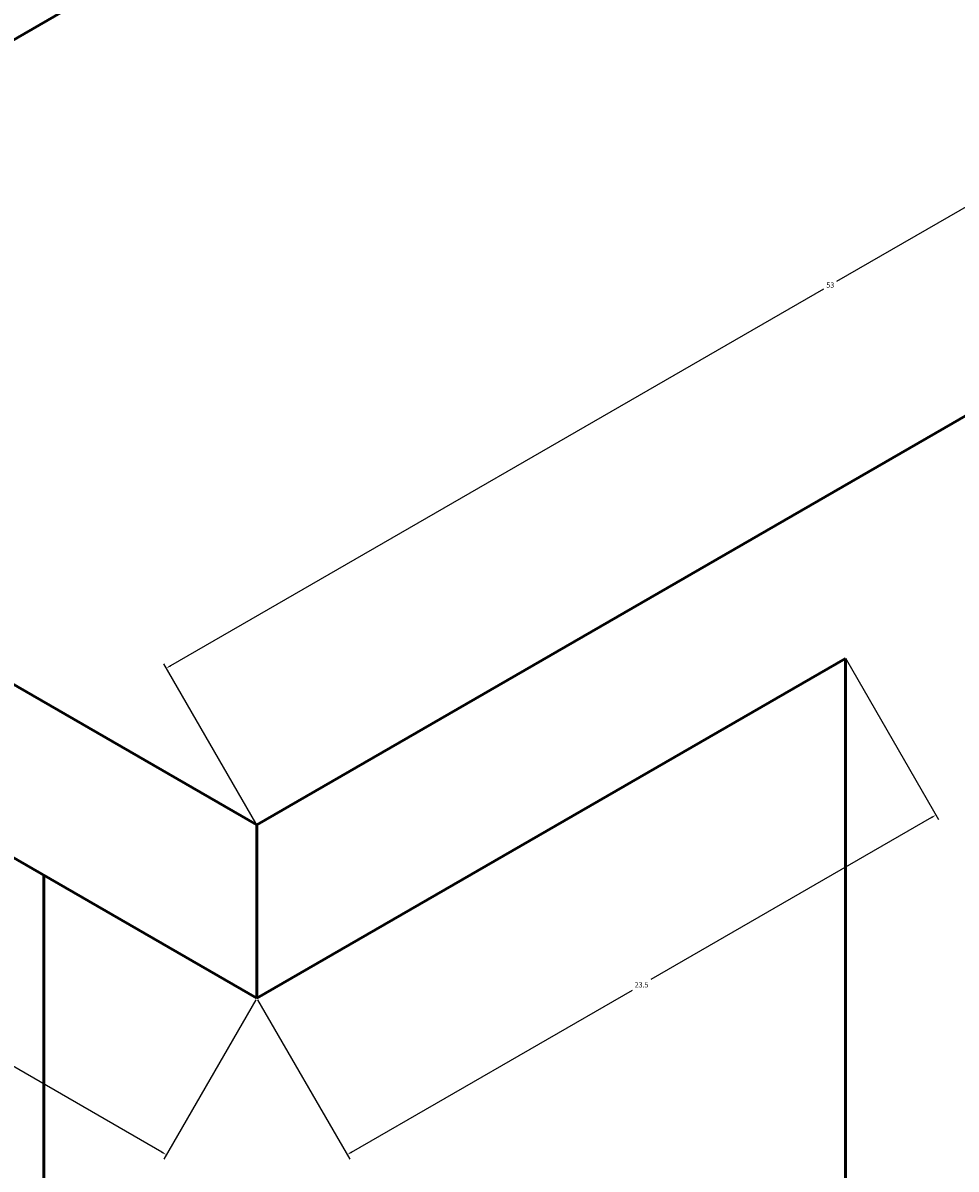
# Model space of a CAD drawing. Units: inches. Extents: x -23 to 69, y -27 to 96.
# Tile 3 of 10: x 8 to 40, y -5 to 35. Entities that reach past the tile are written whole.
import ezdxf

# ---------------------------------------------------------------- set-up
doc = ezdxf.new("R2010")
doc.units = ezdxf.units.IN
doc.header["$MEASUREMENT"] = 0
doc.layers.add('M-DIMS', color=2, linetype='Continuous', lineweight=18)
doc.layers.add('M-OUTL', color=7, linetype='Continuous', lineweight=50)
doc.styles.get("Standard").update_dxf_attribs({"font": 'arial.ttf'})
doc.dimstyles.get("Standard").update_dxf_attribs({"dimtxt": 0.18, "dimasz": 0.18, "dimexe": 0.18, "dimexo": 0.0625, "dimgap": 0.09, "dimtad": 0, "dimtih": 1, "dimtoh": 1, "dimdec": 4, "dimzin": 0, "dimdsep": 46, "dimtxsty": 'Standard', "dimcen": 0.09, "dimadec": 0, "dimazin": 0, "dimtfac": 1, "dimtdec": 4, "dimtofl": 0, "dimtmove": 0, "dimatfit": 3, "dimfxl": 1, "dimtolj": 1, "dimtzin": 0, "dimarcsym": 0})

# ---------------------------------------------------------------- blocks, each defined once
blk = doc.blocks.new('*D1')
at = {"layer": 'Defpoints', "color": 0, "transparency": 16777216}
for p in [(59.046, 39.281), (62.171, 33.869), (16.271, 7.369)]:
    blk.add_point(p, dxfattribs=at)
at = {"layer": 'M-DIMS', "color": 0, "lineweight": -2, "transparency": 16777216}
for p, q in [((62.139, 33.923), (58.956, 39.437)), ((58.89, 39.191), (36.315, 26.158)), ((13.302, 12.871), (35.877, 25.905)), ((16.24, 7.423), (13.056, 12.937))]:
    blk.add_line(p, q, dxfattribs=at)
at = {"layer": 'M-DIMS', "color": 0, "transparency": 16777216}
for points in [[(58.875, 39.217), (58.905, 39.165), (59.046, 39.281)], [(13.287, 12.897), (13.317, 12.845), (13.146, 12.781)]]:
    blk.add_solid(points, dxfattribs=at)
at = {"layer": 'M-DIMS', "color": 0, "transparency": 16777216, "insert": (36.096, 26.031), "char_height": 0.18, "attachment_point": 5}
blk.add_mtext('\\A1;53', dxfattribs=at)
blk = doc.blocks.new('*D2')
at = {"layer": 'Defpoints', "color": 0, "transparency": 16777216}
for p in [(-16.638, 20.369), (-19.763, 14.956), (16.271, 1.369)]:
    blk.add_point(p, dxfattribs=at)
at = {"layer": 'M-DIMS', "color": 0, "lineweight": -2, "transparency": 16777216}
for p, q in [((-16.669, 20.315), (-19.853, 14.8)), ((-19.607, 14.866), (-3.527, 5.582)), ((12.99, -3.954), (-3.089, 5.33)), ((16.24, 1.315), (13.056, -4.2))]:
    blk.add_line(p, q, dxfattribs=at)
at = {"layer": 'M-DIMS', "color": 0, "transparency": 16777216}
for points in [[(-19.592, 14.892), (-19.622, 14.84), (-19.763, 14.956)], [(13.005, -3.928), (12.975, -3.98), (13.146, -4.044)]]:
    blk.add_solid(points, dxfattribs=at)
at = {"layer": 'M-DIMS', "color": 0, "transparency": 16777216, "insert": (-3.308, 5.456), "char_height": 0.18, "attachment_point": 5}
blk.add_mtext('\\A1;38', dxfattribs=at)
blk = doc.blocks.new('*D7')
at = {"layer": 'Defpoints', "color": 0, "transparency": 16777216}
for p in [(36.623, 13.119), (16.271, 1.369), (19.396, -4.044)]:
    blk.add_point(p, dxfattribs=at)
at = {"layer": 'M-DIMS', "color": 0, "lineweight": -2, "transparency": 16777216}
for p, q in [((36.654, 13.065), (39.838, 7.55)), ((39.592, 7.616), (29.887, 2.013)), ((19.552, -3.954), (29.257, 1.649)), ((16.302, 1.315), (19.486, -4.2))]:
    blk.add_line(p, q, dxfattribs=at)
at = {"layer": 'M-DIMS', "color": 0, "transparency": 16777216}
for points in [[(39.577, 7.642), (39.607, 7.59), (39.748, 7.706)], [(19.537, -3.928), (19.567, -3.98), (19.396, -4.044)]]:
    blk.add_solid(points, dxfattribs=at)
at = {"layer": 'M-DIMS', "color": 0, "transparency": 16777216, "insert": (29.572, 1.831), "char_height": 0.18, "attachment_point": 5}
blk.add_mtext('\\A1;23.5', dxfattribs=at)
blk = doc.blocks.new('*D13')
at = {"layer": 'Defpoints', "color": 0, "transparency": 16777216}
for p in [(15.838, 89.119), (-22.888, -20.881), (36.623, -20.881)]:
    blk.add_point(p, dxfattribs=at)
at = {"layer": 'M-DIMS', "color": 0, "lineweight": -2, "transparency": 16777216}
for p, q in [((15.776, 89.119), (-23.068, 89.119)), ((-22.888, 88.939), (-22.888, 34.301)), ((-22.888, -20.701), (-22.888, 33.937)), ((36.56, -20.881), (-23.068, -20.881))]:
    blk.add_line(p, q, dxfattribs=at)
at = {"layer": 'M-DIMS', "color": 0, "transparency": 16777216}
for points in [[(-22.918, 88.939), (-22.858, 88.939), (-22.888, 89.119)], [(-22.918, -20.701), (-22.858, -20.701), (-22.888, -20.881)]]:
    blk.add_solid(points, dxfattribs=at)
at = {"layer": 'M-DIMS', "color": 0, "transparency": 16777216, "insert": (-22.888, 34.119), "char_height": 0.18, "attachment_point": 5}
blk.add_mtext('\\A1;110', dxfattribs=at)
blk = doc.blocks.new('*D17')
at = {"layer": 'Defpoints', "color": 0, "transparency": 16777216}
for p in [(62.171, 27.869), (-16.638, 20.369), (62.171, -27.131)]:
    blk.add_point(p, dxfattribs=at)
at = {"layer": 'M-DIMS', "color": 0, "lineweight": -2, "transparency": 16777216}
for p, q in [((62.171, 27.806), (62.171, -27.311)), ((-16.638, 20.306), (-16.638, -27.311)), ((-16.458, -27.131), (22.391, -27.131)), ((61.991, -27.131), (23.142, -27.131))]:
    blk.add_line(p, q, dxfattribs=at)
at = {"layer": 'M-DIMS', "color": 0, "transparency": 16777216}
for points in [[(-16.458, -27.101), (-16.458, -27.161), (-16.638, -27.131)], [(61.991, -27.101), (61.991, -27.161), (62.171, -27.131)]]:
    blk.add_solid(points, dxfattribs=at)
at = {"layer": 'M-DIMS', "color": 0, "transparency": 16777216, "insert": (22.766, -27.131), "char_height": 0.18, "attachment_point": 5}
blk.add_mtext('\\A1;78.81', dxfattribs=at)

msp = doc.modelspace()

# ---------------------------------------------------------------- linework, layer by layer
at = {"layer": 'M-OUTL'}
for p, q in [((34.4578, 49.8686), (-11.4416, 23.3686)), ((16.2712, 7.3686), (62.1706, 33.8686)), ((-11.4416, 23.3686), (16.2712, 7.3686)), ((-11.4416, 17.3686), (16.2712, 1.3686)), ((16.2712, 1.3686), (36.6228, 13.1186)), ((36.6228, 13.1186), (36.6228, -20.8814)), ((16.2712, 7.3686), (16.2712, 1.3686)), ((8.91, -4.8814), (8.91, 5.6186))]:
    msp.add_line(p, q, dxfattribs=at)

# ---------------------------------------------------------------- dimensions: what is measured, and where the dimension line sits
at = {"layer": 'M-DIMS'}
for base, p1, p2, angle, override, picture, middle in [((-22.8877, -20.8814), (15.8382, 89.1186), (36.6228, -20.8814), 90, {"dimdec": 0, "dimlfac": 1, "dimrnd": 0, "dimzin": 0, "dimdsep": 46, "dimlunit": 2}, '*D13', (-22.8877, 34.1186)), ((59.0456, 39.2813), (16.2712, 7.3686), (62.1706, 33.8686), 30, {"dimdec": 0, "dimlfac": 1, "dimrnd": 0, "dimzin": 0, "dimdsep": 46, "dimlunit": 2}, '*D1', (36.0959, 26.0313)), ((-19.7627, 14.956), (16.2712, 1.3686), (-16.6377, 20.3686), 150, {"dimdec": 0, "dimlfac": 1, "dimrnd": 0, "dimzin": 0, "dimdsep": 46, "dimlunit": 2}, '*D2', (-3.3083, 5.456)), ((19.3962, -4.044), (36.6228, 13.1186), (16.2712, 1.3686), 210, {"dimdec": 1, "dimlfac": 1, "dimrnd": 0, "dimzin": 0, "dimdsep": 46, "dimlunit": 2}, '*D7', (29.572, 1.831))]:
    dim = msp.add_linear_dim(base=base, p1=p1, p2=p2, angle=angle, dimstyle='Standard', override=override, dxfattribs=at)
    dim.commit()
    dim.dimension.update_dxf_attribs({"geometry": picture, "text_midpoint": middle})
dim = msp.add_linear_dim(base=(62.1706, -27.1314), p1=(-16.6377, 20.3686), p2=(62.1706, 27.8686), dimstyle='Standard', override={"dimdec": 2, "dimlfac": 1, "dimrnd": 0, "dimzin": 0, "dimdsep": 46, "dimlunit": 2}, dxfattribs=at)
dim.commit()
dim.dimension.update_dxf_attribs({"geometry": '*D17', "text_midpoint": (22.7664, -27.1314)})

doc.saveas('drawing.dxf')
